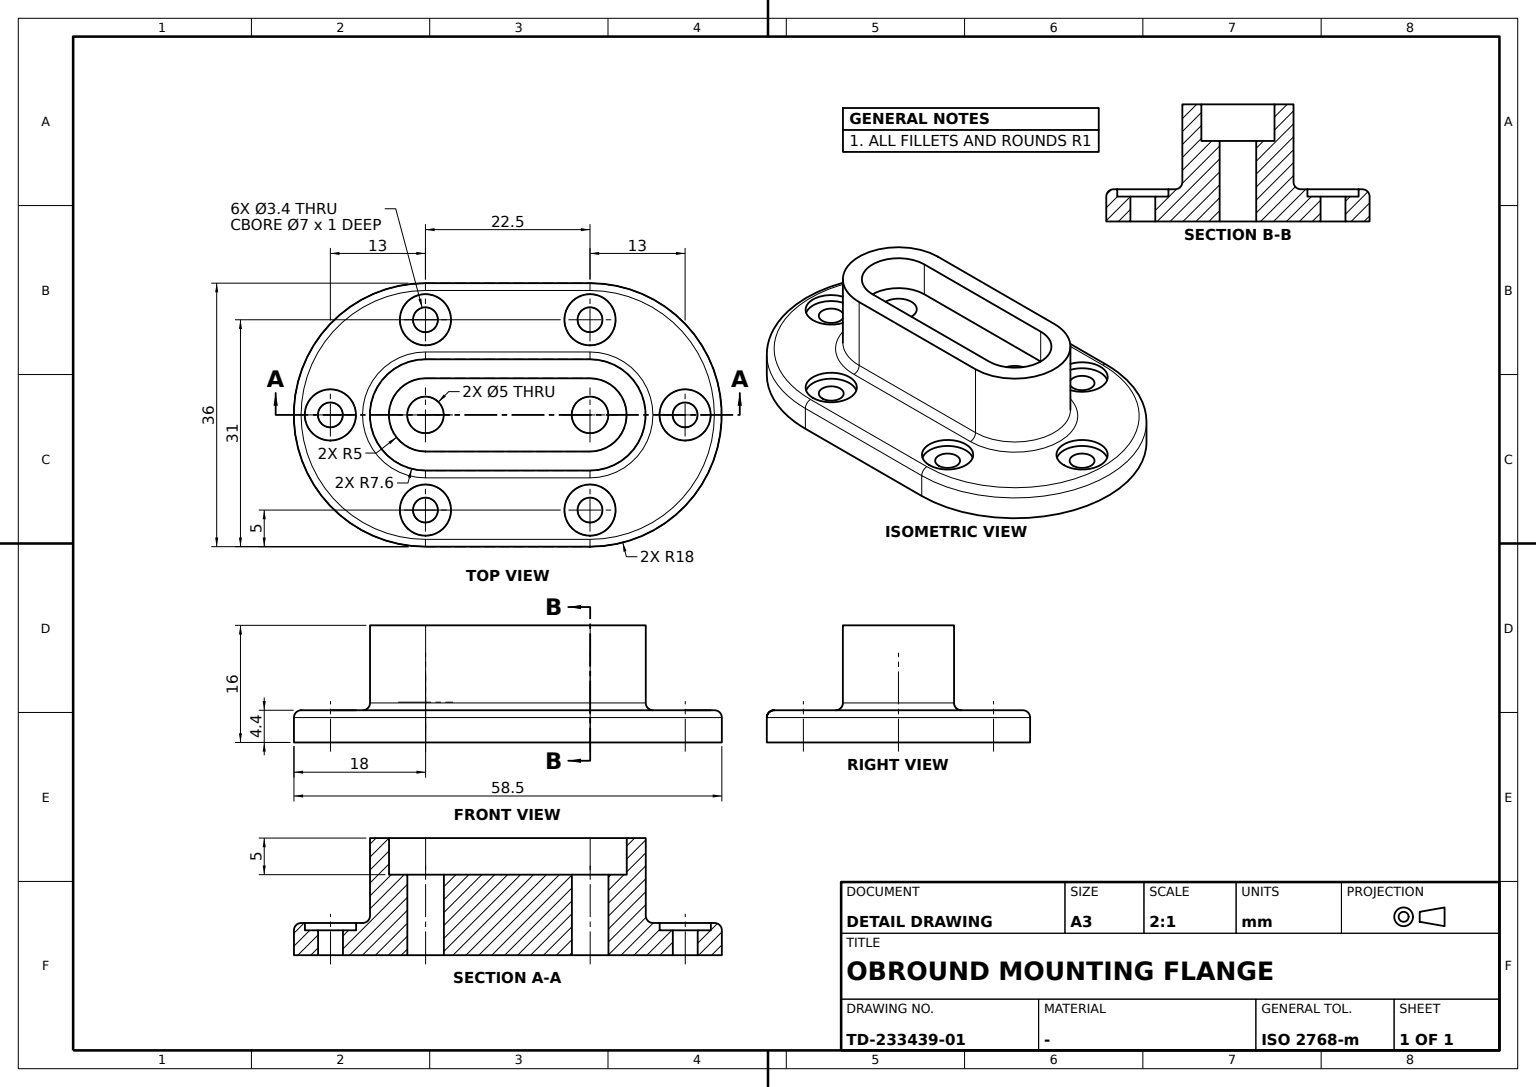
CATIA V5 part; units mm, degrees
sketch "Sketch1" plane through (0, 0, 0) normal (0, 0, 1) x (0, 1, 0)
  arc A0 (-11.25, 18) -> (-11.25, -18) centre (-11.25, 0) ccw
  point P0 (-11.25, 0)
  arc A1 (11.25, -18) -> (11.25, 18) centre (11.25, 0) ccw
  point P1 (11.25, 0)
  point P2 (-11.25, 18)
  line L0 (-11.25, 18) -> (11.25, 18)
  point P3 (11.25, 18)
  point P4 (11.25, -18)
  point P5 (-11.25, -18)
  line L1 (-11.25, -18) -> (11.25, -18)
  dimension "radius A0" = 18
  dimension "length L0" = 22.5
  constraint coincidence P0 x-axis
  constraint coincidence P1 x-axis
  constraint horizontal L0 x-axis
  constraint tangency L0 A0
  constraint symmetry P3 P4 x-axis
  constraint symmetry P2 P5 x-axis
  constraint symmetry L0 L1 x-axis
  constraint symmetry A0 A1 y-axis
extrude "Pad1" add sketch "Sketch1" along normal mid plane 4.4
sketch "Sketch2" plane through (0, 0, 2.2) normal (0, 0, 1) x (0, 1, 0)
  circle A0 centre (-11.25, 13) radius 3.5
  point P0 (-11.25, 13)
  circle A1 centre (-11.25, -13) radius 3.5
  point P1 (-11.25, -13)
  circle A2 centre (-24.25, 0) radius 3.5
  point P2 (-24.25, 0)
  circle A3 centre (11.25, 13) radius 3.5
  circle A4 centre (24.25, 0) radius 3.5
  circle A5 centre (11.25, -13) radius 3.5
  dimension "radius A0" = 3.5
  dimension "distance P0 y axis" = 11.25
  dimension "distance P0 x axis" = 13
  dimension "radius A1" = 3.5
  dimension "radius A2" = 3.5
  dimension "distance P2 y axis" = 24.25
  constraint symmetry P1 P0 x-axis
  constraint symmetry A0 A3 y-axis
  constraint symmetry A2 A4 y-axis
  constraint symmetry A1 A5 y-axis
  constraint coincidence P2 x-axis
extrude "Pocket1" cut sketch "Sketch2" against normal blind 1
sketch "Sketch3" plane through (0, 0, 1.2) normal (0, 0, 1) x (0, 1, 0)
  circle A0 centre (-11.25, 13) radius 1.7
  circle A1 centre (-11.25, 13) radius 3.5 construction
  circle A2 centre (11.25, 13) radius 1.7
  circle A3 centre (24.25, 0) radius 1.7
  point P0 (24.25, 0)
  circle A4 centre (11.25, -13) radius 1.7
  circle A5 centre (24.25, 0) radius 3.5 construction
  circle A6 centre (11.25, -13) radius 3.5 construction
  circle A7 centre (11.25, 13) radius 3.5 construction
  circle A8 centre (-11.25, -13) radius 1.7
  circle A9 centre (-24.25, 0) radius 1.7
  dimension "radius A0" = 1.7
  dimension "radius A3" = 1.7
  dimension "radius A4" = 1.7
  dimension "radius A2" = 1.7
  constraint concentricity A0 A1
  constraint concentricity A3 A5
  constraint concentricity A4 A6
  constraint concentricity A2 A7
  constraint coincidence P0 x-axis
  constraint symmetry A4 A8 y-axis
  constraint symmetry A3 A9 y-axis
extrude "Pocket2" cut sketch "Sketch3" against normal through all
fillet "Fillet1" radius 1 4 edges at (18, 0, 2.2) (0, 29.25, 2.2) (0, -29.25, 2.2) (-18, 0, 2.2)
sketch "Sketch4" plane through (0, 0, 2.2) normal (0, 0, 1) x (0, 1, 0)
  arc A0 (-11.25, 7.6) -> (-11.25, -7.6) centre (-11.25, 0) ccw
  point P0 (-11.25, 0)
  arc A1 (11.25, -7.6) -> (11.25, 7.6) centre (11.25, 0) ccw
  point P1 (11.25, 0)
  arc A2 (11.25, -5) -> (11.25, 5) centre (11.25, 0) ccw
  arc A3 (-11.25, 5) -> (-11.25, -5) centre (-11.25, 0) ccw
  point P2 (-11.25, 7.6)
  line L0 (-11.25, 7.6) -> (11.25, 7.6)
  point P3 (11.25, 7.6)
  point P4 (11.25, -7.6)
  point P5 (-11.25, -7.6)
  line L1 (-11.25, -7.6) -> (11.25, -7.6)
  point P6 (-11.25, 5)
  line L2 (-11.25, 5) -> (11.25, 5)
  point P7 (11.25, 5)
  point P8 (11.25, -5)
  point P9 (-11.25, -5)
  line L3 (-11.25, -5) -> (11.25, -5)
  dimension "radius A1" = 7.6
  dimension "radius A2" = 5
  dimension "radius A0" = 7.6
  dimension "radius A3" = 5
  dimension "distance P0 P1" = 22.5
  constraint coincidence P0 x-axis
  constraint coincidence P1 x-axis
  constraint symmetry P0 P1 y-axis
  constraint symmetry P3 P4 x-axis
  constraint symmetry P2 P5 x-axis
  constraint symmetry L0 L1 x-axis
  constraint symmetry P7 P8 x-axis
  constraint symmetry P6 P9 x-axis
  constraint symmetry L2 L3 x-axis
  constraint horizontal L0 x-axis
  constraint horizontal L2 x-axis
  constraint tangency L0 A0
  constraint tangency L2 A3
extrude "Pad2" add sketch "Sketch4" along normal blind 11.6
sketch "Sketch5" plane through (0, 0, 2.2) normal (0, 0, 1) x (0, 1, 0)
  arc A0 (-11.25, 5) -> (-11.25, -5) centre (-11.25, 0) ccw
  point P0 (-11.25, 0)
  arc A1 (11.25, -5) -> (11.25, 5) centre (11.25, 0) ccw
  point P1 (11.25, 0)
  point P2 (-11.25, 5)
  line L0 (-11.25, 5) -> (11.25, 5)
  point P3 (11.25, 5)
  point P4 (11.25, -5)
  point P5 (-11.25, -5)
  line L1 (-11.25, -5) -> (11.25, -5)
  dimension "radius A0" = 5
  dimension "distance P0 P1" = 22.5
  constraint coincidence P0 x-axis
  constraint coincidence P1 x-axis
  constraint horizontal L0 x-axis
  constraint tangency L0 A0
  constraint tangency L0 A1
  constraint tangency L1 A1
  constraint symmetry P0 P1 y-axis
  constraint symmetry P3 P4 x-axis
  constraint symmetry P2 P5 x-axis
  constraint symmetry L0 L1 x-axis
extrude "Pad3" add sketch "Sketch5" along normal blind 6.6
sketch "Sketch6" plane through (0, 0, 8.8) normal (0, 0, 1) x (0, 1, 0)
  circle A0 centre (-11.25, 0) radius 2.5
  point P0 (-11.25, 0)
  circle A1 centre (11.25, 0) radius 2.5
  point P1 (11.25, 0)
  dimension "radius A1" = 2.5
  dimension "radius A0" = 2.5
  dimension "distance P0 P1" = 22.5
  constraint coincidence P0 x-axis
  constraint coincidence P1 x-axis
  constraint symmetry P0 P1 y-axis
extrude "Pocket3" cut sketch "Sketch6" against normal through all
fillet "Fillet2" radius 1 4 edges at (0, -18.85, 2.2) (7.6, 0, 2.2) (0, 18.85, 2.2) (-7.6, 0, 2.2)
